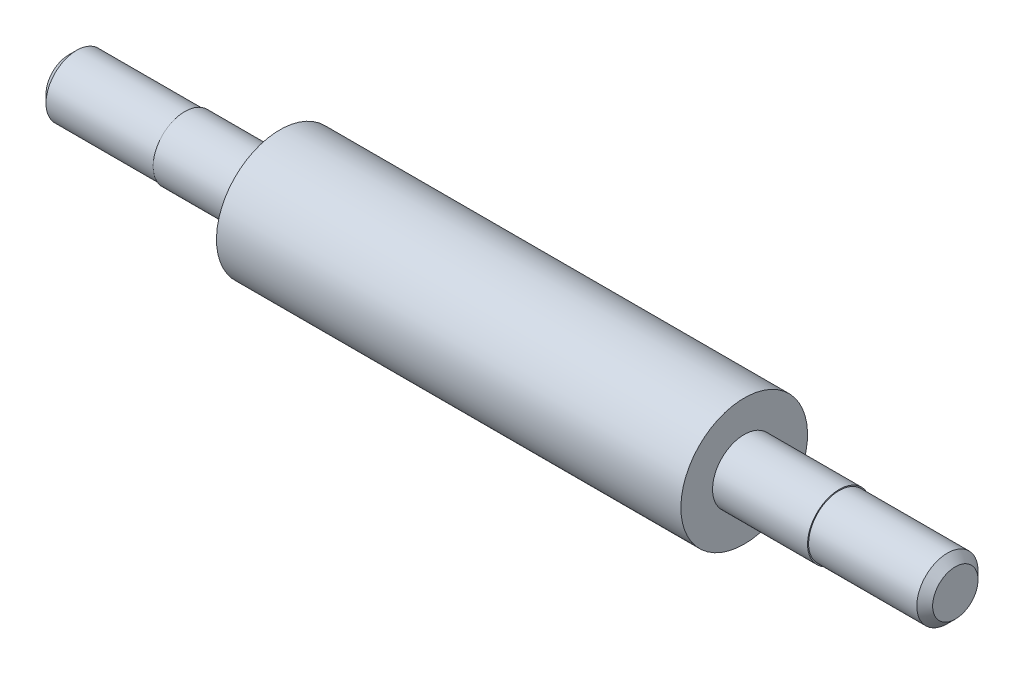
from build123d import *

# Parameters (mm, degrees)
END_CHAMFER_7_5X45_SIZE = 7.5


with BuildPart() as part:
    # Shaft Profile Sketch → Stepped Shaft Body (revolve)
    with BuildSketch(Plane.XY, mode=Mode.PRIVATE) as stepped_shaft_body_sk:
        Polygon((220, 60), (-220, 60), (-220, 30), (-310, 30), (-310, 29), (-420, 29), (-420, 0), (420, 0), (420, 29), (310, 29), (310, 30), (220, 30), align=None)
    revolve(stepped_shaft_body_sk.sketch.rotate(Axis((-420, 0, 0), (1, 0, 0)), 180), axis=Axis((-420, 0, 0), (1, 0, 0)))

    # End Chamfer 7.5x45°
    end_chamfer_7_5x45_edges = [part.edges().sort_by_distance(p)[0] for p in [
        (-420, 29, 0),
        (420, 29, 0),
    ]]
    chamfer(end_chamfer_7_5x45_edges, length=END_CHAMFER_7_5X45_SIZE)


solid = part.part
